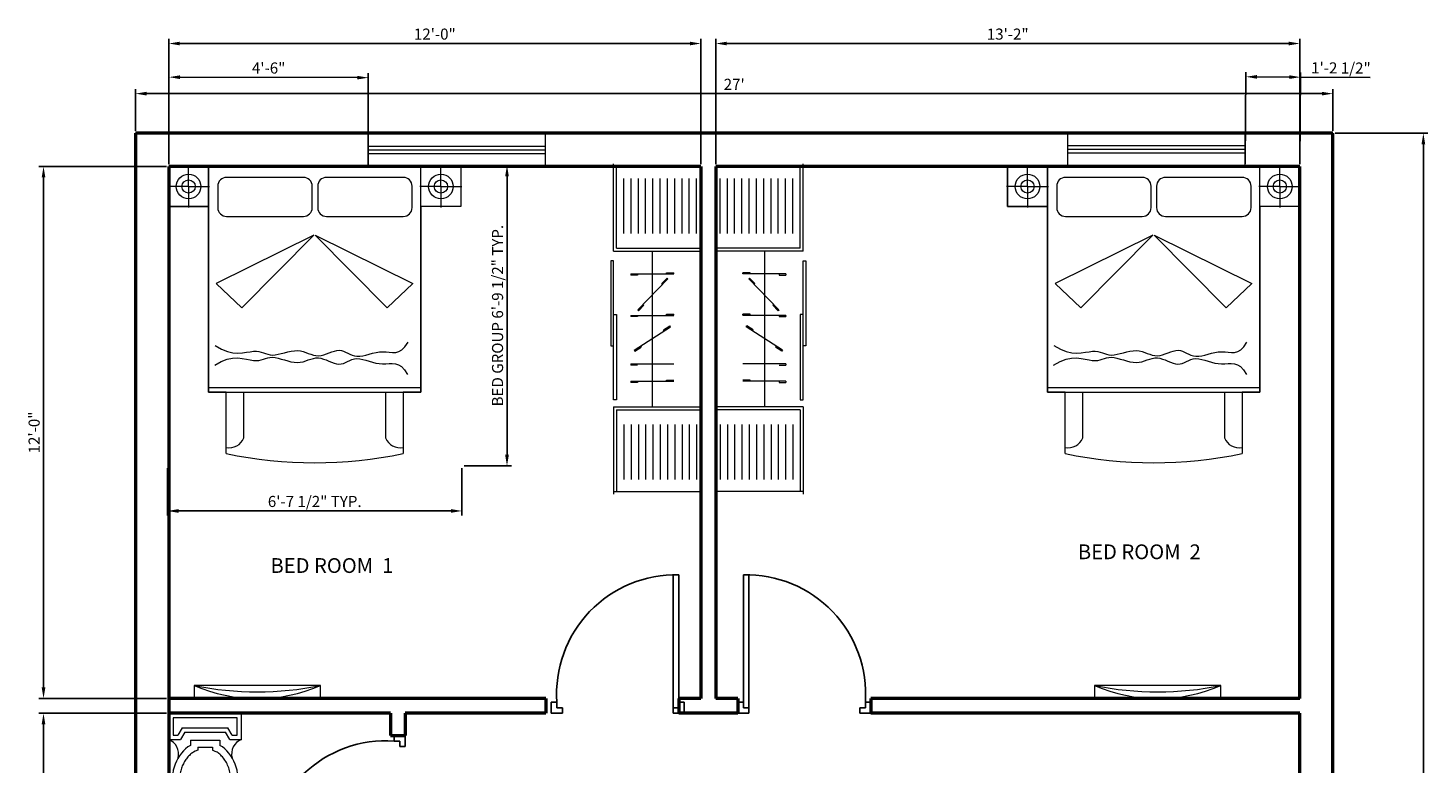
# Model space of a CAD drawing. Units: inches. Extents: x 108 to 1546, y -229 to 513.
# Tile 11 of 11: x 1167 to 1546, y 282 to 481. Entities that reach past the tile are written whole.
import ezdxf

# ---------------------------------------------------------------- set-up
doc = ezdxf.new("R2010")
doc.units = ezdxf.units.IN
for name, color, linetype, lineweight in [('A-ANNO-DIMS', 2, 'Continuous', 18), ('A-AREA-IDEN', 4, 'Continuous', 18), ('A-FLOR-FIXT', 9, 'Continuous', 18), ('A-FURN', 8, 'Continuous', 13), ('door', 1, 'Continuous', 25), ('tv', 2, 'Continuous', 13), ('wall', 7, 'Continuous', 50), ('WINDOW', 212, 'Continuous', 18)]:
    doc.layers.add(name, color=color, linetype=linetype, lineweight=lineweight)
doc.styles.get("Standard").update_dxf_attribs({"font": 'arial.ttf'})
doc.dimstyles.new('ISO-25', dxfattribs={"dimtxt": 3, "dimasz": 3, "dimexe": 1.25, "dimexo": 0.625, "dimtad": 1, "dimdec": 1, "dimlunit": 3, "dimtxsty": 'Standard', "dimcen": 2.5, "dimadec": 0, "dimazin": 0, "dimtfac": 1, "dimtdec": 1, "dimtmove": 0, "dimatfit": 3, "dimfxl": 1, "dimarcsym": 0})

# ---------------------------------------------------------------- blocks, each defined once
blk = doc.blocks.new('A$C4F543DC7')
for p, q in [((0.013, 3.35, -0.169), (3.313, 3.35, -0.169)), ((0.463, 3.35, -0.169), (0.013, 3.35, -0.169)), ((0.013, 2.896, -0.169), (0.013, 3.35, -0.169)), ((0.013, 3.35, -0.169), (0.013, 2.896, -0.169)), ((0.238, 3.123, -0.439), (0.238, 3.361, -0.439)), ((0.463, 3.35, -0.169), (0.463, 0.8, -0.169)), ((2.863, 3.35, -0.169), (0.463, 3.35, -0.169)), ((0.463, 2.896, -0.169), (0.463, 3.35, -0.169)), ((2.863, 0.8, -0.169), (2.863, 3.35, -0.169)), ((2.863, 3.35, -0.169), (3.313, 3.35, -0.169)), ((2.863, 2.896, -0.169), (2.863, 3.35, -0.169)), ((3.089, 3.123, -0.439), (3.089, 3.361, -0.439)), ((3.313, 3.35, -0.169), (3.313, 2.896, -0.169)), ((3.313, 3.35, -0.169), (3.313, 2.896, -0.169)), ((1.535, 3.226, -0.169), (0.668, 3.226, -0.169)), ((2.664, 3.226, -0.169), (1.797, 3.226, -0.169)), ((0.238, 3.123, -0.439), (0, 3.123, -0.439)), ((0.238, 3.123, -0.439), (0.476, 3.123, -0.439)), ((0.238, 3.123, -0.439), (0.238, 2.885, -0.439)), ((0.568, 3.126, -0.169), (0.568, 2.884, -0.169)), ((1.635, 2.884, -0.169), (1.635, 3.126, -0.169)), ((1.697, 3.126, -0.169), (1.697, 2.884, -0.169)), ((2.764, 2.884, -0.169), (2.764, 3.126, -0.169)), ((3.089, 3.123, -0.439), (2.851, 3.123, -0.439)), ((3.089, 3.123, -0.439), (3.089, 2.885, -0.439)), ((3.089, 3.123, -0.439), (3.327, 3.123, -0.439)), ((0.463, 2.896, -0.169), (0.013, 2.896, -0.169)), ((0.013, 2.896, -0.169), (0.463, 2.896, -0.169)), ((0.463, 0.8, -0.169), (0.463, 2.896, -0.169)), ((2.863, 2.896, -0.169), (2.863, 0.8, -0.169)), ((3.313, 2.896, -0.169), (2.863, 2.896, -0.169)), ((3.313, 2.896, -0.169), (2.863, 2.896, -0.169)), ((0.668, 2.784, -0.169), (1.535, 2.784, -0.169)), ((1.797, 2.784, -0.169), (2.664, 2.784, -0.169)), ((1.653, 2.573, -0.169), (0.55, 2.025, -0.169)), ((0.841, 1.752, -0.169), (1.653, 2.573, -0.169)), ((2.481, 1.752, -0.169), (1.669, 2.573, -0.169)), ((1.669, 2.573, -0.169), (2.772, 2.025, -0.169)), ((0.55, 2.025, -0.169), (0.841, 1.752, -0.169)), ((2.772, 2.025, -0.169), (2.481, 1.752, -0.169)), ((0.537, 1.327, -0.169), (0.609, 1.284, -0.169)), ((0.609, 1.284, -0.169), (0.676, 1.257, -0.169)), ((1.396, 1.261, -0.169), (1.433, 1.266, -0.169)), ((1.433, 1.266, -0.169), (1.468, 1.268, -0.169)), ((1.468, 1.268, -0.169), (1.501, 1.264, -0.169)), ((1.885, 1.263, -0.169), (1.913, 1.27, -0.169)), ((1.913, 1.27, -0.169), (1.94, 1.272, -0.169)), ((1.94, 1.272, -0.169), (1.965, 1.269, -0.169)), ((1.965, 1.269, -0.169), (1.989, 1.262, -0.169)), ((2.613, 1.257, -0.169), (2.648, 1.277, -0.169)), ((2.648, 1.277, -0.169), (2.683, 1.312, -0.169)), ((2.683, 1.312, -0.169), (2.718, 1.364, -0.169)), ((0.533, 1.105, -0.169), (0.607, 1.146, -0.169)), ((0.607, 1.146, -0.169), (0.674, 1.171, -0.169)), ((0.674, 1.171, -0.169), (0.736, 1.183, -0.169)), ((0.676, 1.257, -0.169), (0.737, 1.243, -0.169)), ((0.736, 1.183, -0.169), (0.793, 1.185, -0.169)), ((0.737, 1.243, -0.169), (0.794, 1.239, -0.169)), ((0.793, 1.185, -0.169), (0.845, 1.18, -0.169)), ((0.794, 1.239, -0.169), (0.846, 1.242, -0.169)), ((0.845, 1.18, -0.169), (0.891, 1.172, -0.169)), ((0.846, 1.242, -0.169), (0.893, 1.249, -0.169)), ((0.891, 1.172, -0.169), (0.933, 1.163, -0.169)), ((0.893, 1.249, -0.169), (0.935, 1.256, -0.169)), ((0.933, 1.163, -0.169), (0.97, 1.156, -0.169)), ((0.935, 1.256, -0.169), (0.972, 1.261, -0.169)), ((0.97, 1.156, -0.169), (1.003, 1.155, -0.169)), ((0.972, 1.261, -0.169), (1.004, 1.262, -0.169)), ((1.003, 1.155, -0.169), (1.032, 1.158, -0.169)), ((1.004, 1.262, -0.169), (1.033, 1.258, -0.169)), ((1.032, 1.158, -0.169), (1.058, 1.164, -0.169)), ((1.033, 1.258, -0.169), (1.06, 1.251, -0.169)), ((1.058, 1.164, -0.169), (1.083, 1.172, -0.169)), ((1.06, 1.251, -0.169), (1.084, 1.242, -0.169)), ((1.083, 1.172, -0.169), (1.107, 1.18, -0.169)), ((1.084, 1.242, -0.169), (1.108, 1.234, -0.169)), ((1.107, 1.18, -0.169), (1.132, 1.187, -0.169)), ((1.108, 1.234, -0.169), (1.132, 1.226, -0.169)), ((1.132, 1.226, -0.169), (1.158, 1.22, -0.169)), ((1.132, 1.187, -0.169), (1.157, 1.192, -0.169)), ((1.157, 1.192, -0.169), (1.185, 1.193, -0.169)), ((1.158, 1.22, -0.169), (1.185, 1.218, -0.169)), ((1.185, 1.218, -0.169), (1.216, 1.22, -0.169)), ((1.185, 1.193, -0.169), (1.216, 1.19, -0.169)), ((1.216, 1.22, -0.169), (1.25, 1.226, -0.169)), ((1.216, 1.19, -0.169), (1.249, 1.183, -0.169)), ((1.249, 1.183, -0.169), (1.284, 1.173, -0.169)), ((1.25, 1.226, -0.169), (1.285, 1.235, -0.169)), ((1.284, 1.173, -0.169), (1.321, 1.163, -0.169)), ((1.285, 1.235, -0.169), (1.322, 1.244, -0.169)), ((1.321, 1.163, -0.169), (1.358, 1.152, -0.169)), ((1.322, 1.244, -0.169), (1.359, 1.253, -0.169)), ((1.358, 1.152, -0.169), (1.394, 1.143, -0.169)), ((1.359, 1.253, -0.169), (1.396, 1.261, -0.169)), ((1.394, 1.143, -0.169), (1.431, 1.137, -0.169)), ((1.431, 1.137, -0.169), (1.466, 1.135, -0.169)), ((1.466, 1.135, -0.169), (1.499, 1.137, -0.169)), ((1.499, 1.137, -0.169), (1.531, 1.143, -0.169)), ((1.501, 1.264, -0.169), (1.532, 1.257, -0.169)), ((1.531, 1.143, -0.169), (1.561, 1.152, -0.169)), ((1.532, 1.257, -0.169), (1.562, 1.247, -0.169)), ((1.561, 1.152, -0.169), (1.59, 1.162, -0.169)), ((1.562, 1.247, -0.169), (1.591, 1.237, -0.169)), ((1.59, 1.162, -0.169), (1.619, 1.172, -0.169)), ((1.591, 1.237, -0.169), (1.62, 1.226, -0.169)), ((1.619, 1.172, -0.169), (1.648, 1.18, -0.169)), ((1.62, 1.226, -0.169), (1.648, 1.217, -0.169)), ((1.648, 1.217, -0.169), (1.676, 1.211, -0.169)), ((1.648, 1.18, -0.169), (1.676, 1.185, -0.169)), ((1.676, 1.211, -0.169), (1.705, 1.209, -0.169)), ((1.676, 1.185, -0.169), (1.705, 1.186, -0.169)), ((1.705, 1.209, -0.169), (1.735, 1.212, -0.169)), ((1.705, 1.186, -0.169), (1.734, 1.182, -0.169)), ((1.734, 1.182, -0.169), (1.764, 1.173, -0.169)), ((1.735, 1.212, -0.169), (1.765, 1.22, -0.169)), ((1.764, 1.173, -0.169), (1.794, 1.162, -0.169)), ((1.765, 1.22, -0.169), (1.795, 1.23, -0.169)), ((1.794, 1.162, -0.169), (1.824, 1.149, -0.169)), ((1.795, 1.23, -0.169), (1.826, 1.242, -0.169)), ((1.824, 1.149, -0.169), (1.854, 1.137, -0.169)), ((1.826, 1.242, -0.169), (1.856, 1.253, -0.169)), ((1.854, 1.137, -0.169), (1.883, 1.126, -0.169)), ((1.856, 1.253, -0.169), (1.885, 1.263, -0.169)), ((1.883, 1.126, -0.169), (1.911, 1.119, -0.169)), ((1.911, 1.119, -0.169), (1.937, 1.115, -0.169)), ((1.937, 1.115, -0.169), (1.963, 1.118, -0.169)), ((1.963, 1.118, -0.169), (1.987, 1.124, -0.169)), ((1.987, 1.124, -0.169), (2.011, 1.134, -0.169)), ((1.989, 1.262, -0.169), (2.012, 1.251, -0.169)), ((2.011, 1.134, -0.169), (2.034, 1.145, -0.169)), ((2.012, 1.251, -0.169), (2.036, 1.239, -0.169)), ((2.034, 1.145, -0.169), (2.059, 1.157, -0.169)), ((2.036, 1.239, -0.169), (2.06, 1.227, -0.169)), ((2.059, 1.157, -0.169), (2.084, 1.167, -0.169)), ((2.06, 1.227, -0.169), (2.085, 1.216, -0.169)), ((2.084, 1.167, -0.169), (2.111, 1.174, -0.169)), ((2.085, 1.216, -0.169), (2.112, 1.208, -0.169)), ((2.111, 1.174, -0.169), (2.14, 1.177, -0.169)), ((2.112, 1.208, -0.169), (2.141, 1.204, -0.169)), ((2.14, 1.177, -0.169), (2.172, 1.175, -0.169)), ((2.141, 1.204, -0.169), (2.172, 1.205, -0.169)), ((2.172, 1.205, -0.169), (2.206, 1.21, -0.169)), ((2.172, 1.175, -0.169), (2.206, 1.169, -0.169)), ((2.206, 1.21, -0.169), (2.242, 1.218, -0.169)), ((2.206, 1.169, -0.169), (2.241, 1.16, -0.169)), ((2.241, 1.16, -0.169), (2.278, 1.149, -0.169)), ((2.242, 1.218, -0.169), (2.279, 1.228, -0.169)), ((2.278, 1.149, -0.169), (2.316, 1.138, -0.169)), ((2.279, 1.228, -0.169), (2.317, 1.238, -0.169)), ((2.316, 1.138, -0.169), (2.354, 1.128, -0.169)), ((2.317, 1.238, -0.169), (2.356, 1.246, -0.169)), ((2.354, 1.128, -0.169), (2.392, 1.121, -0.169)), ((2.356, 1.246, -0.169), (2.394, 1.253, -0.169)), ((2.392, 1.121, -0.169), (2.43, 1.117, -0.169)), ((2.394, 1.253, -0.169), (2.433, 1.255, -0.169)), ((2.43, 1.117, -0.169), (2.468, 1.118, -0.169)), ((2.433, 1.255, -0.169), (2.47, 1.253, -0.169)), ((2.468, 1.118, -0.169), (2.504, 1.121, -0.169)), ((2.47, 1.253, -0.169), (2.506, 1.249, -0.169)), ((2.504, 1.121, -0.169), (2.54, 1.123, -0.169)), ((2.506, 1.249, -0.169), (2.542, 1.246, -0.169)), ((2.54, 1.123, -0.169), (2.576, 1.12, -0.169)), ((2.542, 1.246, -0.169), (2.578, 1.248, -0.169)), ((2.576, 1.12, -0.169), (2.611, 1.109, -0.169)), ((2.578, 1.248, -0.169), (2.613, 1.257, -0.169)), ((2.611, 1.109, -0.169), (2.645, 1.088, -0.169)), ((2.645, 1.088, -0.169), (2.679, 1.052, -0.169)), ((2.679, 1.052, -0.169), (2.712, 0.999, -0.169)), ((0.463, 0.85, -0.169), (2.863, 0.85, -0.169)), ((0.463, 0.8, -0.169), (2.863, 0.8, -0.169)), ((0.663, 0.8, -0.169), (0.463, 0.8, -0.169)), ((0.663, 0.8, -0.169), (2.663, 0.8, -0.169)), ((0.663, 0.104, -0.169), (0.663, 0.8, -0.169)), ((0.663, 0.104, -0.169), (0.663, 0.8, -0.169)), ((0.863, 0.281, -0.169), (0.863, 0.8, -0.169)), ((2.463, 0.8, -0.169), (2.463, 0.281, -0.169)), ((2.863, 0.8, -0.169), (2.663, 0.8, -0.169)), ((2.663, 0.8, -0.169), (2.663, 0.104, -0.169)), ((2.663, 0.8, -0.169), (2.663, 0.104, -0.169))]:
    blk.add_line(p, q)
for centre, radius in [((0.238, 3.123, -0.439), 0.139), ((0.238, 3.123, -0.439), 0.075), ((3.089, 3.123, -0.439), 0.139), ((3.089, 3.123, -0.439), 0.075)]:
    blk.add_circle(centre, radius)
for centre, radius, start, end in [((0.668, 3.126, -0.169), 0.1, 90, 180), ((1.535, 3.126, -0.169), 0.1, 0, 90), ((1.797, 3.126, -0.169), 0.1, 90, 180), ((2.664, 3.126, -0.169), 0.1, 0, 90), ((0.668, 2.884, -0.169), 0.1, 180, 270), ((1.535, 2.884, -0.169), 0.1, 270, 0), ((1.797, 2.884, -0.169), 0.1, 180, 270), ((2.664, 2.884, -0.169), 0.1, 270, 0), ((0.699, 0.347, -0.169), 0.177, 258.2616, 338.032), ((2.627, 0.347, -0.169), 0.177, 201.968, 281.7384), ((1.663, 4.86, -0.169), 4.86, 258.1252, 281.8748), ((1.663, 4.86, -0.169), 4.86, 258.1252, 281.8748)]:
    blk.add_arc(centre, radius, start, end)
blk = doc.blocks.new('A$C34930FF8')
at = {"ltscale": 0.05}
for p, q in [((0, 2252.4), (0, 16.8)), ((600, 2252.4), (0, 2252.4)), ((185.4, 1513), (185.4, 1521.5)), ((227.1, 1479.2), (233.2, 1485.2)), ((237.7, 1513), (237.7, 1521.5)), ((263.6, 1441.7), (269.7, 1447.7)), ((436.7, 1513), (436.7, 1504.4)), ((482.5, 1513), (482.5, 1504.4)), ((398.2, 1303.6), (392.1, 1297.6)), ((434.8, 1266.1), (428.7, 1260.1)), ((185.4, 1229.1), (185.4, 1237.7)), ((209.5, 1150.1), (214.1, 1157.3)), ((237.7, 1229.1), (237.7, 1237.7)), ((436.7, 1228.2), (436.7, 1219.7)), ((482.5, 1228.2), (482.5, 1219.7)), ((253.5, 1121.8), (258.1, 1129)), ((415.3, 1017.6), (410.6, 1010.5)), ((459.3, 989.3), (454.7, 982.1)), ((482.5, 894.9), (482.5, 886.3)), ((237.7, 775.3), (237.7, 783.9)), ((436.7, 775.3), (436.7, 766.8)), ((482.5, 775.3), (482.5, 766.8)), ((600, 16.8), (0, 16.8))]:
    blk.add_line(p, q, dxfattribs=at)
for p, q in [((580, 1690.9), (580, 2252.4)), ((600, 1669.3), (600, 2269.3)), ((30, 1790.9), (30, 2169.3)), ((80, 1790.9), (80, 2169.3)), ((130, 1790.9), (130, 2169.3)), ((180, 1790.9), (180, 2169.3)), ((230, 1790.9), (230, 2169.3)), ((280, 1790.9), (280, 2169.3)), ((330, 1790.9), (330, 2169.3)), ((380, 1790.9), (380, 2169.3)), ((430, 1790.9), (430, 2169.3)), ((480, 1790.9), (480, 2169.3)), ((530, 1790.9), (530, 2169.3)), ((580, 1690.9), (0, 1690.9)), ((600, 1669.3), (0, 1669.3)), ((335.4, 1666.1), (335.4, 603.1)), ((600, 1603.3), (620, 1603.3)), ((600, 1018.7), (600, 1603.3)), ((620, 1603.3), (620, 1018.7)), ((237.7, 1521.5), (185.4, 1521.5)), ((482.5, 1513), (185.4, 1513)), ((434.8, 1266.1), (227.4, 1478.9)), ((269.7, 1447.7), (233.2, 1485.2)), ((436.7, 1504.4), (482.5, 1504.4)), ((428.7, 1260.1), (392.1, 1297.6)), ((237.7, 1237.7), (185.4, 1237.7)), ((482.5, 1228.2), (185.4, 1228.2)), ((258.1, 1129), (214.1, 1157.3)), ((436.7, 1219.7), (482.5, 1219.7)), ((600, 1233.4), (580, 1233.4)), ((580, 1233.4), (580, 648.7)), ((600, 648.7), (600, 1233.4)), ((459.3, 989.3), (209.5, 1150.1)), ((454.7, 982.1), (410.6, 1010.5)), ((620, 1018.7), (600, 1018.7)), ((482.5, 894.9), (185.4, 894.9)), ((436.7, 886.3), (482.5, 886.3)), ((237.7, 783.9), (185.4, 783.9)), ((482.5, 775.3), (185.4, 775.3)), ((436.7, 766.8), (482.5, 766.8)), ((600, 600), (0, 600)), ((580, 578.3), (0, 578.3)), ((580, 648.7), (600, 648.7)), ((580, 578.3), (580, 16.8)), ((600, 600), (600, 0)), ((30, 478.3), (30, 100)), ((80, 478.3), (80, 100)), ((130, 478.3), (130, 100)), ((180, 478.3), (180, 100)), ((230, 478.3), (230, 100)), ((280, 478.3), (280, 100)), ((330, 478.3), (330, 100)), ((380, 478.3), (380, 100)), ((430, 478.3), (430, 100)), ((480, 478.3), (480, 100)), ((530, 478.3), (530, 100))]:
    blk.add_line(p, q)
blk = doc.blocks.new('A$C7C8779AE')
for p, q in [((0, 0.7405), (0, 0.5605)), ((0.5, 0.7405), (0, 0.7405)), ((0.47, 0.7105), (0.03, 0.7105)), ((0.03, 0.7105), (0.03, 0.5905)), ((0.47, 0.5905), (0.47, 0.7105)), ((0.5, 0.5605), (0.5, 0.7405)), ((0.03, 0.5905), (0.063, 0.5905)), ((0.093, 0.6405), (0.063, 0.5905)), ((0.11, 0.6105), (0.08, 0.5605)), ((0.093, 0.6405), (0.407, 0.6405)), ((0.11, 0.6105), (0.39, 0.6105)), ((0.42, 0.5605), (0.39, 0.6105)), ((0.437, 0.5905), (0.407, 0.6405)), ((0.437, 0.5905), (0.47, 0.5905)), ((0, 0.5605), (0.08, 0.5605)), ((0.1497, 0.557), (0.1497, 0.5203)), ((0.1497, 0.557), (0.3514, 0.557)), ((0.1997, 0.507), (0.1997, 0.4879)), ((0.1997, 0.507), (0.3014, 0.507)), ((0.3014, 0.507), (0.3014, 0.4879)), ((0.3514, 0.557), (0.3514, 0.5203)), ((0.42, 0.5605), (0.5, 0.5605))]:
    blk.add_line(p, q)
for centre, start, end in [((-0.0386, 0.4613), 344.64203, 68.73386), ((0.5386, 0.4613), 111.26614, 195.35797)]:
    blk.add_arc(centre, 0.1064, start, end)
blk.add_ellipse((0.2506, 0.2744), major_axis=(0, 0.2744), ratio=0.828948, start_param=0.459479, end_param=5.823706)
blk.add_open_spline([(0.1997, 0.4879), (0.1697, 0.474), (0.1642, 0.4702), (0.1512, 0.4602), (0.1438, 0.4535), (0.1298, 0.4388), (0.1233, 0.4306), (0.1111, 0.4131), (0.1055, 0.4037), (0.0956, 0.3838), (0.0912, 0.3733), (0.0838, 0.3516), (0.0808, 0.3403), (0.0762, 0.3172), (0.0746, 0.3055), (0.073, 0.2817), (0.0729, 0.2698), (0.0743, 0.246), (0.0758, 0.2342), (0.0801, 0.2111), (0.0831, 0.1998), (0.0903, 0.1779), (0.0945, 0.1673), (0.1043, 0.1473), (0.1098, 0.1378), (0.1218, 0.12), (0.1283, 0.1118), (0.1421, 0.0968), (0.1494, 0.09), (0.1646, 0.078), (0.1725, 0.0728), (0.1887, 0.064), (0.1969, 0.0603), (0.2137, 0.0547), (0.2222, 0.0527), (0.2392, 0.0502), (0.2478, 0.0498), (0.2664, 0.0505), (0.2764, 0.052), (0.2963, 0.0573), (0.3061, 0.061), (0.3253, 0.0707), (0.3346, 0.0766), (0.3525, 0.0906), (0.3611, 0.0987), (0.3771, 0.1169), (0.3845, 0.127), (0.3978, 0.1488), (0.4037, 0.1605), (0.4137, 0.1853), (0.4178, 0.1983), (0.424, 0.2251), (0.4261, 0.2389), (0.4282, 0.2668), (0.4283, 0.2809), (0.4262, 0.3088), (0.4241, 0.3226), (0.418, 0.3495), (0.414, 0.3625), (0.404, 0.3873), (0.3982, 0.3991), (0.385, 0.421), (0.3776, 0.4311), (0.3617, 0.4494), (0.3531, 0.4575), (0.3382, 0.4693), (0.3321, 0.4736), (0.3014, 0.4879)], degree=3, knots=[0.459479, 0.459479, 0.459479, 0.459479, 0.567422, 0.567422, 0.720865, 0.720865, 0.874307, 0.874307, 1.02775, 1.02775, 1.181192, 1.181192, 1.334635, 1.334635, 1.488077, 1.488077, 1.64152, 1.64152, 1.794963, 1.794963, 1.948405, 1.948405, 2.101848, 2.101848, 2.25529, 2.25529, 2.408733, 2.408733, 2.562175, 2.562175, 2.715618, 2.715618, 2.86906, 2.86906, 3.022503, 3.022503, 3.175946, 3.175946, 3.356457, 3.356457, 3.536968, 3.536968, 3.717479, 3.717479, 3.89799, 3.89799, 4.078501, 4.078501, 4.259012, 4.259012, 4.439523, 4.439523, 4.620035, 4.620035, 4.800546, 4.800546, 4.981057, 4.981057, 5.161568, 5.161568, 5.342079, 5.342079, 5.52259, 5.52259, 5.703101, 5.703101, 5.823706, 5.823706, 5.823706, 5.823706])
blk = doc.blocks.new('*D25')
at = {"layer": 'A-ANNO-DIMS', "color": 0, "lineweight": -2, "transparency": 16777216}
for p, q in [((1195.94, 453.09), (1195.94, 464.41)), ((1198.94, 463.16), (1516.94, 463.16)), ((1519.94, 453.09), (1519.94, 464.41))]:
    blk.add_line(p, q, dxfattribs=at)
at = {"layer": 'A-ANNO-DIMS', "color": 0, "transparency": 16777216}
for points in [[(1198.94, 463.66), (1198.94, 462.66), (1195.94, 463.16)], [(1516.94, 463.66), (1516.94, 462.66), (1519.94, 463.16)]]:
    blk.add_solid(points, dxfattribs=at)
at = {"layer": 'Defpoints', "color": 0, "transparency": 16777216}
for p in [(1519.94, 463.16), (1195.94, 452.47), (1519.94, 452.47)]:
    blk.add_point(p, dxfattribs=at)
at = {"layer": 'A-ANNO-DIMS', "color": 0, "transparency": 16777216, "insert": (1357.94, 465.29), "char_height": 3, "attachment_point": 5}
blk.add_mtext("27'", dxfattribs=at)
blk = doc.blocks.new('*D26')
at = {"layer": 'A-ANNO-DIMS', "color": 0, "lineweight": -2, "transparency": 16777216}
for p, q in [((1520.57, 452.47), (1545.65, 452.47)), ((1544.4, 449.47), (1544.4, -0.53)), ((1520.57, -3.53), (1545.65, -3.53))]:
    blk.add_line(p, q, dxfattribs=at)
at = {"layer": 'A-ANNO-DIMS', "color": 0, "transparency": 16777216}
for points in [[(1543.9, 449.47), (1544.9, 449.47), (1544.4, 452.47)], [(1543.9, -0.53), (1544.9, -0.53), (1544.4, -3.53)]]:
    blk.add_solid(points, dxfattribs=at)
at = {"layer": 'Defpoints', "color": 0, "transparency": 16777216}
for p in [(1519.94, 452.47), (1519.94, -3.53), (1544.4, -3.53)]:
    blk.add_point(p, dxfattribs=at)
at = {"layer": 'A-ANNO-DIMS', "color": 0, "transparency": 16777216, "insert": (1542.24, 224.47), "char_height": 3, "attachment_point": 5, "rotation": 90}
blk.add_mtext("38'", dxfattribs=at)
blk = doc.blocks.new('WINDOW-48X9')
for p, q in [((0, 9), (0, 0)), ((0, 9), (48, 9)), ((48, 9), (48, 0)), ((0, 5.5), (48, 5.5)), ((0, 4.5), (48, 4.5)), ((0, 3.5), (48, 3.5)), ((0, 0), (48, 0))]:
    blk.add_line(p, q)
blk = doc.blocks.new('DOOR-SWING-36')
for p, q in [((1.5, 1.5), (1.5, 37.5)), ((3, 1.5), (3, 37.5)), ((0, 3), (0, 0)), ((1.5, 3), (0, 3)), ((1.5, 1.5), (1.5, 3)), ((3, 1.5), (1.5, 1.5)), ((3, 0), (3, 1.5)), ((33, 0), (33, 1.5)), ((33, 1.5), (34.5, 1.5)), ((34.5, 1.5), (34.5, 3)), ((34.5, 3), (36, 3)), ((36, 3), (36, 0)), ((0, 0), (3, 0)), ((36, 0), (33, 0))]:
    blk.add_line(p, q)
blk.add_arc((2.25, 5.18), 32.32, 356.1244, 91.3295)
blk = doc.blocks.new('TV-WALL-MOUNT')
blk.add_lwpolyline([(0, 0), (34.19, 0), (34.19, 3.56), (0, 3.56)], close=True)
for centre, radius, start, end in [((17.1, 42.8), 42.8, 246.4582, 293.5418), ((17.1, 84.72), 82.93, 258.1036, 281.8964)]:
    blk.add_arc(centre, radius, start, end)
blk = doc.blocks.new('*D40')
at = {"layer": 'A-ANNO-DIMS', "color": 0, "lineweight": -2, "transparency": 16777216}
for p, q in [((1284.9, 443.74), (1297.72, 443.74)), ((1296.47, 365.43), (1296.47, 440.74)), ((1284.9, 362.43), (1297.72, 362.43))]:
    blk.add_line(p, q, dxfattribs=at)
at = {"layer": 'A-ANNO-DIMS', "color": 0, "transparency": 16777216}
for points in [[(1295.97, 440.74), (1296.97, 440.74), (1296.47, 443.74)], [(1295.97, 365.43), (1296.97, 365.43), (1296.47, 362.43)]]:
    blk.add_solid(points, dxfattribs=at)
at = {"layer": 'Defpoints', "color": 0, "transparency": 16777216}
for p in [(1284.28, 443.74), (1296.47, 443.74), (1284.28, 362.43)]:
    blk.add_point(p, dxfattribs=at)
at = {"layer": 'A-ANNO-DIMS', "color": 0, "transparency": 16777216, "insert": (1294.3, 403.09), "char_height": 3, "attachment_point": 5, "rotation": 90}
blk.add_mtext('BED GROUP 6\'-9 1/2" TYP.', dxfattribs=at)
blk = doc.blocks.new('*D41')
at = {"layer": 'A-ANNO-DIMS', "color": 0, "lineweight": -2, "transparency": 16777216}
for p, q in [((1204.62, 361.8), (1204.62, 348.98)), ((1284.28, 361.8), (1284.28, 348.98)), ((1207.62, 350.23), (1281.28, 350.23))]:
    blk.add_line(p, q, dxfattribs=at)
at = {"layer": 'A-ANNO-DIMS', "color": 0, "transparency": 16777216}
for points in [[(1207.62, 350.73), (1207.62, 349.73), (1204.62, 350.23)], [(1281.28, 350.73), (1281.28, 349.73), (1284.28, 350.23)]]:
    blk.add_solid(points, dxfattribs=at)
at = {"layer": 'Defpoints', "color": 0, "transparency": 16777216}
for p in [(1204.62, 362.43), (1284.28, 362.43), (1284.28, 350.23)]:
    blk.add_point(p, dxfattribs=at)
at = {"layer": 'A-ANNO-DIMS', "color": 0, "transparency": 16777216, "insert": (1244.45, 352.41), "char_height": 3, "attachment_point": 5}
blk.add_mtext('6\'-7 1/2" TYP.', dxfattribs=at)
blk = doc.blocks.new('*D101')
at = {"layer": 'A-ANNO-DIMS', "color": 0, "lineweight": -2, "transparency": 16777216}
for p, q in [((1204.94, 444.09), (1204.94, 477.97)), ((1348.94, 444.09), (1348.94, 477.97)), ((1207.94, 476.72), (1345.94, 476.72))]:
    blk.add_line(p, q, dxfattribs=at)
at = {"layer": 'A-ANNO-DIMS', "color": 0, "transparency": 16777216}
for points in [[(1207.94, 477.22), (1207.94, 476.22), (1204.94, 476.72)], [(1345.94, 477.22), (1345.94, 476.22), (1348.94, 476.72)]]:
    blk.add_solid(points, dxfattribs=at)
at = {"layer": 'Defpoints', "color": 0, "transparency": 16777216}
for p in [(1348.94, 476.72), (1204.94, 443.47), (1348.94, 443.47)]:
    blk.add_point(p, dxfattribs=at)
at = {"layer": 'A-ANNO-DIMS', "color": 0, "transparency": 16777216, "insert": (1276.94, 478.88), "char_height": 3, "attachment_point": 5}
blk.add_mtext('12\'-0"', dxfattribs=at)
blk = doc.blocks.new('*D102')
at = {"layer": 'A-ANNO-DIMS', "color": 0, "lineweight": -2, "transparency": 16777216}
for p, q in [((1352.94, 444.09), (1352.94, 477.97)), ((1510.94, 444.09), (1510.94, 477.97)), ((1355.94, 476.72), (1507.94, 476.72))]:
    blk.add_line(p, q, dxfattribs=at)
at = {"layer": 'A-ANNO-DIMS', "color": 0, "transparency": 16777216}
for points in [[(1355.94, 477.22), (1355.94, 476.22), (1352.94, 476.72)], [(1507.94, 477.22), (1507.94, 476.22), (1510.94, 476.72)]]:
    blk.add_solid(points, dxfattribs=at)
at = {"layer": 'Defpoints', "color": 0, "transparency": 16777216}
for p in [(1510.94, 476.72), (1352.94, 443.47), (1510.94, 443.47)]:
    blk.add_point(p, dxfattribs=at)
at = {"layer": 'A-ANNO-DIMS', "color": 0, "transparency": 16777216, "insert": (1431.94, 478.88), "char_height": 3, "attachment_point": 5}
blk.add_mtext('13\'-2"', dxfattribs=at)
blk = doc.blocks.new('*D105')
at = {"layer": 'A-ANNO-DIMS', "color": 0, "lineweight": -2, "transparency": 16777216}
for p, q in [((1204.32, 443.47), (1169.82, 443.47)), ((1171.07, 440.47), (1171.07, 302.47)), ((1204.32, 299.47), (1169.82, 299.47))]:
    blk.add_line(p, q, dxfattribs=at)
at = {"layer": 'A-ANNO-DIMS', "color": 0, "transparency": 16777216}
for points in [[(1170.57, 440.47), (1171.57, 440.47), (1171.07, 443.47)], [(1170.57, 302.47), (1171.57, 302.47), (1171.07, 299.47)]]:
    blk.add_solid(points, dxfattribs=at)
at = {"layer": 'Defpoints', "color": 0, "transparency": 16777216}
for p in [(1204.94, 443.47), (1171.07, 299.47), (1204.94, 299.47)]:
    blk.add_point(p, dxfattribs=at)
at = {"layer": 'A-ANNO-DIMS', "color": 0, "transparency": 16777216, "insert": (1168.92, 371.47), "char_height": 3, "attachment_point": 5, "rotation": 90}
blk.add_mtext('12\'-0"', dxfattribs=at)
blk = doc.blocks.new('*D106')
at = {"layer": 'A-ANNO-DIMS', "color": 0, "lineweight": -2, "transparency": 16777216}
for p, q in [((1204.32, 295.47), (1169.82, 295.47)), ((1171.07, 292.47), (1171.07, 214.47)), ((1204.32, 211.47), (1169.82, 211.47))]:
    blk.add_line(p, q, dxfattribs=at)
at = {"layer": 'A-ANNO-DIMS', "color": 0, "transparency": 16777216}
for points in [[(1170.57, 292.47), (1171.57, 292.47), (1171.07, 295.47)], [(1170.57, 214.47), (1171.57, 214.47), (1171.07, 211.47)]]:
    blk.add_solid(points, dxfattribs=at)
at = {"layer": 'Defpoints', "color": 0, "transparency": 16777216}
for p in [(1204.94, 295.47), (1171.07, 211.47), (1204.94, 211.47)]:
    blk.add_point(p, dxfattribs=at)
at = {"layer": 'A-ANNO-DIMS', "color": 0, "transparency": 16777216, "insert": (1168.92, 253.47), "char_height": 3, "attachment_point": 5, "rotation": 90}
blk.add_mtext('7\'-0"', dxfattribs=at)
blk = doc.blocks.new('*D111')
at = {"layer": 'A-ANNO-DIMS', "color": 0, "lineweight": -2, "transparency": 16777216}
for p, q in [((1204.94, 444.09), (1205.01, 468.87)), ((1208, 467.61), (1255.94, 467.49)), ((1258.88, 443.96), (1258.95, 468.73))]:
    blk.add_line(p, q, dxfattribs=at)
at = {"layer": 'A-ANNO-DIMS', "color": 0, "transparency": 16777216}
for points in [[(1208, 468.11), (1208, 467.11), (1205, 467.62)], [(1255.94, 467.99), (1255.94, 466.99), (1258.94, 467.48)]]:
    blk.add_solid(points, dxfattribs=at)
at = {"layer": 'Defpoints', "color": 0, "transparency": 16777216}
for p in [(1258.94, 467.48), (1204.94, 443.47), (1258.88, 443.33)]:
    blk.add_point(p, dxfattribs=at)
at = {"layer": 'A-ANNO-DIMS', "color": 0, "transparency": 16777216, "insert": (1231.98, 469.71), "char_height": 3, "attachment_point": 5, "rotation": 359.8536}
blk.add_mtext('4\'-6"', dxfattribs=at)
blk = doc.blocks.new('*D112')
at = {"layer": 'A-ANNO-DIMS', "color": 0, "lineweight": -2, "transparency": 16777216}
for p, q in [((1496.22, 444.2), (1496.39, 468.97)), ((1499.38, 467.7), (1508.11, 467.64)), ((1510.94, 444.09), (1511.12, 468.87)), ((1511.11, 467.62), (1530.04, 467.49))]:
    blk.add_line(p, q, dxfattribs=at)
at = {"layer": 'A-ANNO-DIMS', "color": 0, "transparency": 16777216}
for points in [[(1499.38, 468.2), (1499.37, 467.2), (1496.38, 467.72)], [(1508.11, 468.14), (1508.1, 467.14), (1511.11, 467.62)]]:
    blk.add_solid(points, dxfattribs=at)
at = {"layer": 'Defpoints', "color": 0, "transparency": 16777216}
for p in [(1511.11, 467.62), (1496.21, 443.57), (1510.94, 443.47)]:
    blk.add_point(p, dxfattribs=at)
at = {"layer": 'A-ANNO-DIMS', "color": 0, "transparency": 16777216, "insert": (1522.09, 469.72), "char_height": 3, "attachment_point": 5, "rotation": 359.6039}
blk.add_mtext('1\'-2 1/2"', dxfattribs=at)

msp = doc.modelspace()

# ---------------------------------------------------------------- linework, layer by layer
at = {"layer": 'wall'}
for p, q in [((1519.94, 452.47), (1195.94, 452.47)), ((1195.94, 452.47), (1195.94, -3.53)), ((1519.94, -3.53), (1519.94, 452.47)), ((1204.94, 443.47), (1204.94, 5.47)), ((1348.94, 443.47), (1204.94, 443.47)), ((1348.94, 443.47), (1348.94, 299.47)), ((1510.94, 443.47), (1352.94, 443.47)), ((1352.94, 443.47), (1352.94, 299.47)), ((1510.94, 299.47), (1510.94, 443.47)), ((1306.94, 299.47), (1204.94, 299.47)), ((1306.94, 299.47), (1306.94, 295.47)), ((1348.94, 299.47), (1342.94, 299.47)), ((1342.94, 299.47), (1342.94, 295.47)), ((1358.94, 299.47), (1352.94, 299.47)), ((1358.94, 299.47), (1358.94, 295.47)), ((1510.94, 299.47), (1394.94, 299.47)), ((1394.94, 299.47), (1394.94, 295.47)), ((1264.94, 295.47), (1204.94, 295.47)), ((1264.94, 295.47), (1264.94, 289.47)), ((1268.94, 295.47), (1268.94, 289.47)), ((1306.94, 295.47), (1268.94, 295.47)), ((1358.94, 295.47), (1342.94, 295.47)), ((1510.94, 295.47), (1394.94, 295.47)), ((1510.94, 111.47), (1510.94, 295.47)), ((1264.94, 289.47), (1268.94, 289.47))]:
    msp.add_line(p, q, dxfattribs=at)

# ---------------------------------------------------------------- block references
at = {"layer": 'A-FLOR-FIXT', "xscale": 39.37007874015748, "yscale": 39.37007874015748, "zscale": 39.37007874015748}
msp.add_blockref('A$C7C8779AE', (1204.94, 266.32), dxfattribs=at)
at = {"layer": 'A-FURN'}
for name, p, xscale, yscale, zscale in [('A$C4F543DC7', (1204.62, 363.26, 4.04), 23.94379789781286, 23.94379789781286, 23.94379789781286), ('A$C34930FF8', (1348.94, 354.79), -0.0393700787401575, 0.0393700787401575, 0.0393700787401575), ('A$C34930FF8', (1352.94, 354.79), 0.0393700787401575, 0.0393700787401575, 0.0393700787401575), ('A$C4F543DC7', (1431.6, 363.26, 4.04), 23.94379789781286, 23.94379789781286, 23.94379789781286)]:
    msp.add_blockref(name, p, dxfattribs=dict(at, xscale=xscale, yscale=yscale, zscale=zscale))
at = {"layer": 'door', "extrusion": (0, 0, -1), "zscale": -1}
msp.add_blockref('DOOR-SWING-36', (-1344.44, 295.47), dxfattribs=at)
at = {"layer": 'door'}
msp.add_blockref('DOOR-SWING-36', (1358.94, 295.47), dxfattribs=at)
at = {"layer": 'door', "rotation": 90.00000000000006}
msp.add_blockref('DOOR-SWING-36', (1268.94, 253.47), dxfattribs=at)
at = {"layer": 'tv'}
for p in [(1211.82, 299.47), (1455.43, 299.47)]:
    msp.add_blockref('TV-WALL-MOUNT', p, dxfattribs=at)
at = {"layer": 'WINDOW', "rotation": 180}
for p in [(1306.88, 452.33), (1496.21, 452.57)]:
    msp.add_blockref('WINDOW-48X9', p, dxfattribs=at)

# ---------------------------------------------------------------- texts
at = {"layer": 'A-AREA-IDEN', "char_height": 4, "attachment_point": 1}
for s, insert in [('BED ROOM  2', (1450.93, 341.18)), ('BED ROOM  1', (1232.48, 337.46))]:
    msp.add_mtext_dynamic_manual_height_columns(s, width=57.4311, gutter_width=12.5, heights=[12.84], dxfattribs=dict(at, insert=insert))

# ---------------------------------------------------------------- dimensions: what is measured, and where the dimension line sits
at = {"layer": 'A-ANNO-DIMS'}
for base, p1, p2, override, picture, middle in [((1348.94, 476.72), (1204.94, 443.47), (1348.94, 443.47), {"dimdec": 1, "dimlfac": 1, "dimrnd": 0, "dimzin": 1, "dimdsep": 46, "dimlunit": 4, "dimfrac": 2}, '*D101', (1276.94, 478.88)), ((1510.94, 476.72), (1352.94, 443.47), (1510.94, 443.47), {"dimdec": 1, "dimlfac": 1, "dimrnd": 0, "dimzin": 1, "dimdsep": 46, "dimlunit": 4, "dimfrac": 2}, '*D102', (1431.94, 478.88)), ((1519.94, 463.16), (1195.94, 452.47), (1519.94, 452.47), {"dimclrd": 0, "dimclre": 0, "dimclrt": 0}, '*D25', (1357.94, 465.29))]:
    dim = msp.add_linear_dim(base=base, p1=p1, p2=p2, dimstyle='ISO-25', override=override, dxfattribs=at)
    dim.commit()
    dim.dimension.update_dxf_attribs({"geometry": picture, "text_midpoint": middle})
for base, p1, p2, angle, override, picture, middle in [((1511.11, 467.62), (1496.21, 443.57), (1510.94, 443.47), 359.6039, {"dimdec": 1, "dimlfac": 1, "dimrnd": 0, "dimzin": 1, "dimdsep": 46, "dimlunit": 4, "dimfrac": 2}, '*D112', (1522.09, 469.72)), ((1258.94, 467.48), (1204.94, 443.47), (1258.88, 443.33), 359.8536, {"dimdec": 1, "dimlfac": 1, "dimrnd": 0, "dimzin": 1, "dimdsep": 46, "dimlunit": 4, "dimfrac": 2}, '*D111', (1231.98, 469.71)), ((1544.4, -3.53), (1519.94, 452.47), (1519.94, -3.53), 90, {"dimclrd": 0, "dimclre": 0, "dimclrt": 0}, '*D26', (1542.24, 224.47)), ((1171.07, 299.47), (1204.94, 443.47), (1204.94, 299.47), 90, {"dimdec": 1, "dimlfac": 1, "dimrnd": 0, "dimzin": 1, "dimdsep": 46, "dimlunit": 4, "dimfrac": 2}, '*D105', (1168.92, 371.47)), ((1171.07, 211.47), (1204.94, 295.47), (1204.94, 211.47), 90, {"dimdec": 1, "dimlfac": 1, "dimrnd": 0, "dimzin": 1, "dimdsep": 46, "dimlunit": 4, "dimfrac": 2}, '*D106', (1168.92, 253.47))]:
    dim = msp.add_linear_dim(base=base, p1=p1, p2=p2, angle=angle, dimstyle='ISO-25', override=override, dxfattribs=at)
    dim.commit()
    dim.dimension.update_dxf_attribs({"geometry": picture, "text_midpoint": middle})
dim = msp.add_linear_dim(base=(1296.47, 443.74), p1=(1284.28, 362.43), p2=(1284.28, 443.74), angle=90, text='BED GROUP <> TYP.', dimstyle='ISO-25', override={"dimdec": 1, "dimlfac": 1, "dimrnd": 0, "dimzin": 1, "dimdsep": 46, "dimlunit": 4, "dimfrac": 2}, dxfattribs=at)
dim.commit()
dim.dimension.update_dxf_attribs({"geometry": '*D40', "text_midpoint": (1294.3, 403.09)})
dim = msp.add_linear_dim(base=(1284.28, 350.23), p1=(1204.62, 362.43), p2=(1284.28, 362.43), text='<> TYP.', dimstyle='ISO-25', override={"dimdec": 1, "dimlfac": 1, "dimrnd": 0, "dimzin": 1, "dimdsep": 46, "dimlunit": 4, "dimfrac": 2}, dxfattribs=at)
dim.commit()
dim.dimension.update_dxf_attribs({"geometry": '*D41', "text_midpoint": (1244.45, 352.41)})

doc.saveas('drawing.dxf')
